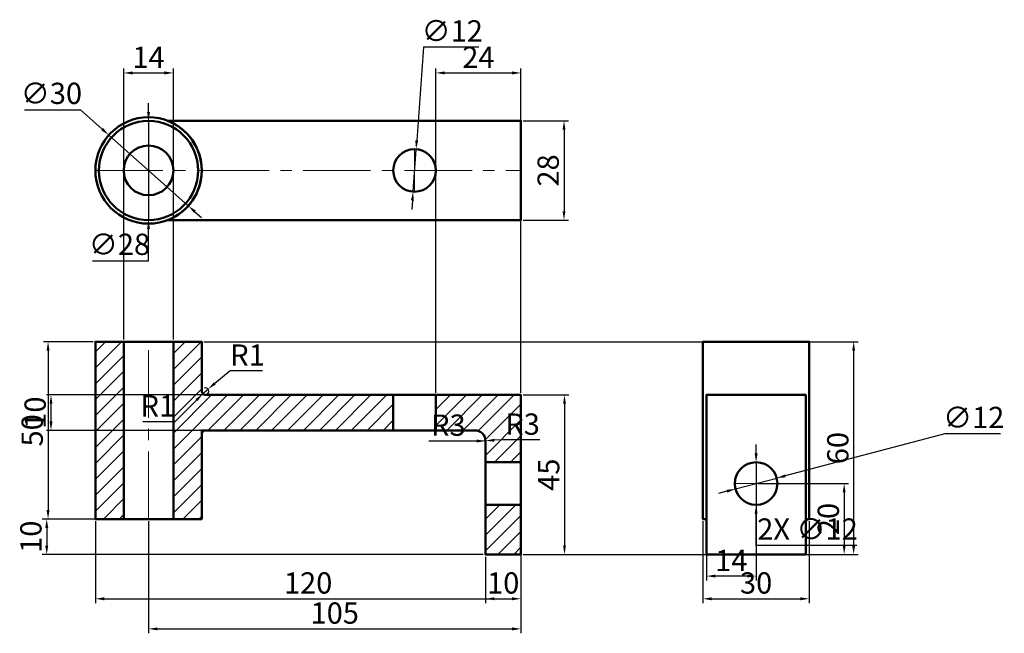
# Model space of a CAD drawing. Units: millimetres. Extents: x 11 to 289, y -7 to 166.
import ezdxf

# ---------------------------------------------------------------- set-up
doc = ezdxf.new("R2010")
doc.units = ezdxf.units.MM
doc.linetypes.add('CENTER2', pattern=[28.575, 19.05, -3.175, 3.175, -3.175])
for name, color, linetype, lineweight in [('M-CNTR', 4, 'CENTER2', 18), ('M-DIMS', 2, 'Continuous', 25), ('M-HATC', 8, 'Continuous', 18), ('M-OUTL', 7, 'Continuous', 50)]:
    doc.layers.add(name, color=color, linetype=linetype, lineweight=lineweight)
doc.styles.get("Standard").update_dxf_attribs({"font": 'arial.ttf'})
doc.dimstyles.new('ISO-25', dxfattribs={"dimtxt": 6, "dimasz": 2.5, "dimexe": 1.25, "dimexo": 0.625, "dimtad": 1, "dimtoh": 1, "dimdec": 0, "dimtxsty": 'Standard', "dimcen": 2.5, "dimadec": 0, "dimazin": 0, "dimtfac": 1, "dimtdec": 0, "dimtmove": 0, "dimatfit": 3, "dimfxl": 1, "dimarcsym": 0})

# ---------------------------------------------------------------- blocks, each defined once
blk = doc.blocks.new('*D1')
at = {"layer": 'Defpoints', "color": 0, "transparency": 16777216}
for p in [(139.29, 47.57), (142.29, 47.57)]:
    blk.add_point(p, dxfattribs=at)
at = {"layer": 'M-DIMS', "color": 0, "lineweight": -2, "transparency": 16777216}
blk.add_line((126.36, 47.57), (139.79, 47.57), dxfattribs=at)
at = {"layer": 'M-DIMS', "color": 0, "transparency": 16777216}
blk.add_solid([(139.79, 47.99), (139.79, 47.15), (142.29, 47.57)], dxfattribs=at)
at = {"layer": 'M-DIMS', "color": 0, "transparency": 16777216, "insert": (131.83, 51.26), "char_height": 6, "attachment_point": 5}
blk.add_mtext('R3', dxfattribs=at)
blk = doc.blocks.new('*D2')
at = {"layer": 'Defpoints', "color": 0, "transparency": 16777216}
for p in [(63.29, 61.57), (64.06, 62.21)]:
    blk.add_point(p, dxfattribs=at)
at = {"layer": 'M-DIMS', "color": 0, "lineweight": -2, "transparency": 16777216}
for p, q in [((70.31, 67.39), (65.98, 63.8)), ((79.45, 67.39), (70.31, 67.39)), ((63.29, 61.57), (64.06, 62.21))]:
    blk.add_line(p, q, dxfattribs=at)
blk.add_arc((63.29, 61.57), 1, 305.8099, 111.2749, dxfattribs=at)
at = {"layer": 'M-DIMS', "color": 0, "transparency": 16777216}
blk.add_solid([(65.72, 64.12), (66.25, 63.48), (64.06, 62.21)], dxfattribs=at)
at = {"layer": 'M-DIMS', "color": 0, "transparency": 16777216, "insert": (75.19, 71.03), "char_height": 6, "attachment_point": 5}
blk.add_mtext('R1', dxfattribs=at)
blk = doc.blocks.new('*D3')
at = {"layer": 'Defpoints', "color": 0, "transparency": 16777216}
for p in [(47.29, 25.57), (152.29, 25.57), (152.29, -5.41)]:
    blk.add_point(p, dxfattribs=at)
at = {"layer": 'M-DIMS', "color": 0, "lineweight": -2, "transparency": 16777216}
for p, q in [((47.29, 24.95), (47.29, -6.66)), ((152.29, 24.95), (152.29, -6.66)), ((49.79, -5.41), (149.79, -5.41))]:
    blk.add_line(p, q, dxfattribs=at)
at = {"layer": 'M-DIMS', "color": 0, "transparency": 16777216}
for points in [[(49.79, -5), (49.79, -5.83), (47.29, -5.41)], [(149.79, -5), (149.79, -5.83), (152.29, -5.41)]]:
    blk.add_solid(points, dxfattribs=at)
at = {"layer": 'M-DIMS', "color": 0, "transparency": 16777216, "insert": (99.79, -1.73), "char_height": 6, "attachment_point": 5}
blk.add_mtext('105', dxfattribs=at)
blk = doc.blocks.new('*D4')
at = {"layer": 'Defpoints', "color": 0, "transparency": 16777216}
for p in [(62.29, 25.57), (18.59, 15.57), (142.29, 15.57)]:
    blk.add_point(p, dxfattribs=at)
at = {"layer": 'M-DIMS', "color": 0, "lineweight": -2, "transparency": 16777216}
for p, q in [((61.66, 25.57), (17.34, 25.57)), ((18.59, 23.07), (18.59, 18.07)), ((141.66, 15.57), (17.34, 15.57))]:
    blk.add_line(p, q, dxfattribs=at)
at = {"layer": 'M-DIMS', "color": 0, "transparency": 16777216}
for points in [[(18.17, 23.07), (19.01, 23.07), (18.59, 25.57)], [(18.17, 18.07), (19.01, 18.07), (18.59, 15.57)]]:
    blk.add_solid(points, dxfattribs=at)
at = {"layer": 'M-DIMS', "color": 0, "transparency": 16777216, "insert": (14.9, 20.57), "char_height": 6, "attachment_point": 5, "rotation": 90}
blk.add_mtext('10', dxfattribs=at)
blk = doc.blocks.new('*D5')
at = {"layer": 'Defpoints', "color": 0, "transparency": 16777216}
for p in [(32.29, 75.57), (18.96, 25.57), (32.29, 25.57)]:
    blk.add_point(p, dxfattribs=at)
at = {"layer": 'M-DIMS', "color": 0, "lineweight": -2, "transparency": 16777216}
for p, q in [((31.66, 75.57), (17.71, 75.57)), ((18.96, 73.07), (18.96, 28.07)), ((31.66, 25.57), (17.71, 25.57))]:
    blk.add_line(p, q, dxfattribs=at)
at = {"layer": 'M-DIMS', "color": 0, "transparency": 16777216}
for points in [[(18.54, 73.07), (19.38, 73.07), (18.96, 75.57)], [(18.54, 28.07), (19.38, 28.07), (18.96, 25.57)]]:
    blk.add_solid(points, dxfattribs=at)
at = {"layer": 'M-DIMS', "color": 0, "transparency": 16777216, "insert": (15.27, 50.57), "char_height": 6, "attachment_point": 5, "rotation": 90}
blk.add_mtext('50', dxfattribs=at)
blk = doc.blocks.new('*D6')
at = {"layer": 'Defpoints', "color": 0, "transparency": 16777216}
for p in [(152.29, 60.57), (152.29, 15.57), (164.57, 15.57)]:
    blk.add_point(p, dxfattribs=at)
at = {"layer": 'M-DIMS', "color": 0, "lineweight": -2, "transparency": 16777216}
for p, q in [((152.91, 60.57), (165.82, 60.57)), ((164.57, 58.07), (164.57, 18.07)), ((152.91, 15.57), (165.82, 15.57))]:
    blk.add_line(p, q, dxfattribs=at)
at = {"layer": 'M-DIMS', "color": 0, "transparency": 16777216}
for points in [[(164.15, 58.07), (164.98, 58.07), (164.57, 60.57)], [(164.15, 18.07), (164.98, 18.07), (164.57, 15.57)]]:
    blk.add_solid(points, dxfattribs=at)
at = {"layer": 'M-DIMS', "color": 0, "transparency": 16777216, "insert": (160.89, 38.07), "char_height": 6, "attachment_point": 5, "rotation": 90}
blk.add_mtext('45', dxfattribs=at)
blk = doc.blocks.new('*D7')
at = {"layer": 'Defpoints', "color": 0, "transparency": 16777216}
for p in [(204.59, 35.57), (218.59, 35.57), (204.59, 9.47)]:
    blk.add_point(p, dxfattribs=at)
at = {"layer": 'M-DIMS', "color": 0, "lineweight": -2, "transparency": 16777216}
for p, q in [((204.59, 34.95), (204.59, 8.22)), ((218.59, 34.95), (218.59, 8.22)), ((216.09, 9.47), (207.09, 9.47))]:
    blk.add_line(p, q, dxfattribs=at)
at = {"layer": 'M-DIMS', "color": 0, "transparency": 16777216}
for points in [[(207.09, 9.89), (207.09, 9.06), (204.59, 9.47)], [(216.09, 9.89), (216.09, 9.06), (218.59, 9.47)]]:
    blk.add_solid(points, dxfattribs=at)
at = {"layer": 'M-DIMS', "color": 0, "transparency": 16777216, "insert": (211.59, 13.11), "char_height": 6, "attachment_point": 5}
blk.add_mtext('14', dxfattribs=at)
blk = doc.blocks.new('*D8')
at = {"layer": 'Defpoints', "color": 0, "transparency": 16777216}
for p in [(218.59, 35.57), (218.59, 15.57), (243.41, 15.57)]:
    blk.add_point(p, dxfattribs=at)
at = {"layer": 'M-DIMS', "color": 0, "lineweight": -2, "transparency": 16777216}
for p, q in [((219.21, 35.57), (244.66, 35.57)), ((243.41, 33.07), (243.41, 18.07)), ((219.21, 15.57), (244.66, 15.57))]:
    blk.add_line(p, q, dxfattribs=at)
at = {"layer": 'M-DIMS', "color": 0, "transparency": 16777216}
for points in [[(243, 33.07), (243.83, 33.07), (243.41, 35.57)], [(243, 18.07), (243.83, 18.07), (243.41, 15.57)]]:
    blk.add_solid(points, dxfattribs=at)
at = {"layer": 'M-DIMS', "color": 0, "transparency": 16777216, "insert": (239.72, 25.57), "char_height": 6, "attachment_point": 5, "rotation": 90}
blk.add_mtext('20', dxfattribs=at)
blk = doc.blocks.new('*D9')
at = {"layer": 'Defpoints', "color": 0, "transparency": 16777216}
for p in [(152.29, 137.87), (152.29, 109.87), (164.43, 109.87)]:
    blk.add_point(p, dxfattribs=at)
at = {"layer": 'M-DIMS', "color": 0, "lineweight": -2, "transparency": 16777216}
for p, q in [((152.91, 137.87), (165.68, 137.87)), ((164.43, 135.37), (164.43, 112.37)), ((152.91, 109.87), (165.68, 109.87))]:
    blk.add_line(p, q, dxfattribs=at)
at = {"layer": 'M-DIMS', "color": 0, "transparency": 16777216}
for points in [[(164.01, 135.37), (164.84, 135.37), (164.43, 137.87)], [(164.01, 112.37), (164.84, 112.37), (164.43, 109.87)]]:
    blk.add_solid(points, dxfattribs=at)
at = {"layer": 'M-DIMS', "color": 0, "transparency": 16777216, "insert": (160.74, 123.87), "char_height": 6, "attachment_point": 5, "rotation": 90}
blk.add_mtext('28', dxfattribs=at)
blk = doc.blocks.new('*D10')
at = {"layer": 'Defpoints', "color": 0, "transparency": 16777216}
for p in [(122.72, 129.86), (121.86, 117.89)]:
    blk.add_point(p, dxfattribs=at)
at = {"layer": 'M-DIMS', "color": 0, "lineweight": -2, "transparency": 16777216}
for p, q in [((124.77, 158.59), (122.89, 132.35)), ((140.45, 158.59), (124.77, 158.59)), ((121.86, 117.89), (122.72, 129.86)), ((121.68, 115.39), (121.5, 112.9))]:
    blk.add_line(p, q, dxfattribs=at)
at = {"layer": 'M-DIMS', "color": 0, "transparency": 16777216}
for points in [[(122.48, 132.38), (123.31, 132.32), (122.72, 129.86)], [(121.27, 115.42), (122.1, 115.36), (121.86, 117.89)]]:
    blk.add_solid(points, dxfattribs=at)
at = {"layer": 'M-DIMS', "color": 0, "transparency": 16777216, "insert": (132.92, 162.45), "char_height": 6, "attachment_point": 5}
blk.add_mtext('∅12', dxfattribs=at)
blk = doc.blocks.new('*D11')
at = {"layer": 'Defpoints', "color": 0, "transparency": 16777216}
for p in [(224.39, 37.1), (212.78, 34.04)]:
    blk.add_point(p, dxfattribs=at)
at = {"layer": 'M-DIMS', "color": 0, "lineweight": -2, "transparency": 16777216}
for p, q in [((271.77, 49.58), (226.81, 37.73)), ((287.46, 49.58), (271.77, 49.58)), ((212.78, 34.04), (224.39, 37.1)), ((210.37, 33.41), (207.95, 32.77))]:
    blk.add_line(p, q, dxfattribs=at)
at = {"layer": 'M-DIMS', "color": 0, "transparency": 16777216}
for points in [[(226.7, 38.14), (226.91, 37.33), (224.39, 37.1)], [(210.26, 33.81), (210.47, 33), (212.78, 34.04)]]:
    blk.add_solid(points, dxfattribs=at)
at = {"layer": 'M-DIMS', "color": 0, "transparency": 16777216, "insert": (279.93, 53.43), "char_height": 6, "attachment_point": 5}
blk.add_mtext('∅12', dxfattribs=at)
blk = doc.blocks.new('*D12')
at = {"layer": 'Defpoints', "color": 0, "transparency": 16777216}
for p in [(36.09, 133.85), (58.49, 113.9)]:
    blk.add_point(p, dxfattribs=at)
at = {"layer": 'M-DIMS', "color": 0, "lineweight": -2, "transparency": 16777216}
for p, q in [((12.36, 140.97), (28.08, 140.97)), ((28.08, 140.97), (34.22, 135.51)), ((58.49, 113.9), (36.09, 133.85)), ((60.36, 112.23), (62.23, 110.57))]:
    blk.add_line(p, q, dxfattribs=at)
at = {"layer": 'M-DIMS', "color": 0, "transparency": 16777216}
for points in [[(34.5, 135.82), (33.94, 135.2), (36.09, 133.85)], [(60.64, 112.54), (60.08, 111.92), (58.49, 113.9)]]:
    blk.add_solid(points, dxfattribs=at)
at = {"layer": 'M-DIMS', "color": 0, "transparency": 16777216, "insert": (19.91, 144.83), "char_height": 6, "attachment_point": 5}
blk.add_mtext('∅30', dxfattribs=at)
blk = doc.blocks.new('*D13')
at = {"layer": 'Defpoints', "color": 0, "transparency": 16777216}
for p in [(32.29, 25.57), (152.29, 15.57), (152.29, 3.07)]:
    blk.add_point(p, dxfattribs=at)
at = {"layer": 'M-DIMS', "color": 0, "lineweight": -2, "transparency": 16777216}
for p, q in [((32.29, 24.95), (32.29, 1.82)), ((152.29, 14.95), (152.29, 1.82)), ((34.79, 3.07), (149.79, 3.07))]:
    blk.add_line(p, q, dxfattribs=at)
at = {"layer": 'M-DIMS', "color": 0, "transparency": 16777216}
for points in [[(34.79, 3.49), (34.79, 2.65), (32.29, 3.07)], [(149.79, 3.49), (149.79, 2.65), (152.29, 3.07)]]:
    blk.add_solid(points, dxfattribs=at)
at = {"layer": 'M-DIMS', "color": 0, "transparency": 16777216, "insert": (92.29, 6.76), "char_height": 6, "attachment_point": 5}
blk.add_mtext('120', dxfattribs=at)
blk = doc.blocks.new('*D14')
at = {"layer": 'Defpoints', "color": 0, "transparency": 16777216}
for p in [(62.29, 75.57), (152.29, 15.57), (246.09, 15.57)]:
    blk.add_point(p, dxfattribs=at)
at = {"layer": 'M-DIMS', "color": 0, "lineweight": -2, "transparency": 16777216}
for p, q in [((62.91, 75.57), (247.34, 75.57)), ((246.09, 73.07), (246.09, 18.07)), ((152.91, 15.57), (247.34, 15.57))]:
    blk.add_line(p, q, dxfattribs=at)
at = {"layer": 'M-DIMS', "color": 0, "transparency": 16777216}
for points in [[(245.67, 73.07), (246.5, 73.07), (246.09, 75.57)], [(245.67, 18.07), (246.5, 18.07), (246.09, 15.57)]]:
    blk.add_solid(points, dxfattribs=at)
at = {"layer": 'M-DIMS', "color": 0, "transparency": 16777216, "insert": (242.4, 45.57), "char_height": 6, "attachment_point": 5, "rotation": 90}
blk.add_mtext('60', dxfattribs=at)
blk = doc.blocks.new('*D15')
at = {"layer": 'Defpoints', "color": 0, "transparency": 16777216}
for p in [(152.29, 151.37), (128.29, 60.57), (152.29, 60.57)]:
    blk.add_point(p, dxfattribs=at)
at = {"layer": 'M-DIMS', "color": 0, "lineweight": -2, "transparency": 16777216}
for p, q in [((128.29, 61.2), (128.29, 152.62)), ((130.79, 151.37), (149.79, 151.37)), ((152.29, 61.2), (152.29, 152.62))]:
    blk.add_line(p, q, dxfattribs=at)
at = {"layer": 'M-DIMS', "color": 0, "transparency": 16777216}
for points in [[(130.79, 151.79), (130.79, 150.95), (128.29, 151.37)], [(149.79, 151.79), (149.79, 150.95), (152.29, 151.37)]]:
    blk.add_solid(points, dxfattribs=at)
at = {"layer": 'M-DIMS', "color": 0, "transparency": 16777216, "insert": (140.29, 155.01), "char_height": 6, "attachment_point": 5}
blk.add_mtext('24', dxfattribs=at)
blk = doc.blocks.new('*D16')
at = {"layer": 'Defpoints', "color": 0, "transparency": 16777216}
for p in [(54.29, 151.37), (40.29, 75.57), (54.29, 75.57)]:
    blk.add_point(p, dxfattribs=at)
at = {"layer": 'M-DIMS', "color": 0, "lineweight": -2, "transparency": 16777216}
for p, q in [((40.29, 76.2), (40.29, 152.62)), ((42.79, 151.37), (51.79, 151.37)), ((54.29, 76.2), (54.29, 152.62))]:
    blk.add_line(p, q, dxfattribs=at)
at = {"layer": 'M-DIMS', "color": 0, "transparency": 16777216}
for points in [[(42.79, 151.79), (42.79, 150.95), (40.29, 151.37)], [(51.79, 151.79), (51.79, 150.95), (54.29, 151.37)]]:
    blk.add_solid(points, dxfattribs=at)
at = {"layer": 'M-DIMS', "color": 0, "transparency": 16777216, "insert": (47.29, 155.01), "char_height": 6, "attachment_point": 5}
blk.add_mtext('14', dxfattribs=at)
blk = doc.blocks.new('*D17')
at = {"layer": 'Defpoints', "color": 0, "transparency": 16777216}
for p in [(203.59, 25.57), (233.59, 25.57), (233.59, 3.07)]:
    blk.add_point(p, dxfattribs=at)
at = {"layer": 'M-DIMS', "color": 0, "lineweight": -2, "transparency": 16777216}
for p, q in [((203.59, 24.95), (203.59, 1.82)), ((233.59, 24.95), (233.59, 1.82)), ((206.09, 3.07), (231.09, 3.07))]:
    blk.add_line(p, q, dxfattribs=at)
at = {"layer": 'M-DIMS', "color": 0, "transparency": 16777216}
for points in [[(206.09, 3.49), (206.09, 2.65), (203.59, 3.07)], [(231.09, 3.49), (231.09, 2.65), (233.59, 3.07)]]:
    blk.add_solid(points, dxfattribs=at)
at = {"layer": 'M-DIMS', "color": 0, "transparency": 16777216, "insert": (218.59, 6.76), "char_height": 6, "attachment_point": 5}
blk.add_mtext('30', dxfattribs=at)
blk = doc.blocks.new('*D18')
at = {"layer": 'Defpoints', "color": 0, "transparency": 16777216}
for p in [(116.29, 60.57), (19.79, 50.57), (116.29, 50.57)]:
    blk.add_point(p, dxfattribs=at)
at = {"layer": 'M-DIMS', "color": 0, "lineweight": -2, "transparency": 16777216}
for p, q in [((115.66, 60.57), (18.54, 60.57)), ((19.79, 58.07), (19.79, 53.07)), ((115.66, 50.57), (18.54, 50.57))]:
    blk.add_line(p, q, dxfattribs=at)
at = {"layer": 'M-DIMS', "color": 0, "transparency": 16777216}
for points in [[(19.37, 58.07), (20.2, 58.07), (19.79, 60.57)], [(19.37, 53.07), (20.2, 53.07), (19.79, 50.57)]]:
    blk.add_solid(points, dxfattribs=at)
at = {"layer": 'M-DIMS', "color": 0, "transparency": 16777216, "insert": (16.1, 55.57), "char_height": 6, "attachment_point": 5, "rotation": 90}
blk.add_mtext('10', dxfattribs=at)
blk = doc.blocks.new('*D19')
at = {"layer": 'Defpoints', "color": 0, "transparency": 16777216}
for p in [(142.29, 15.57), (152.29, 15.57), (152.29, 3.07)]:
    blk.add_point(p, dxfattribs=at)
at = {"layer": 'M-DIMS', "color": 0, "lineweight": -2, "transparency": 16777216}
for p, q in [((142.29, 14.95), (142.29, 1.82)), ((152.29, 14.95), (152.29, 1.82)), ((144.79, 3.07), (149.79, 3.07))]:
    blk.add_line(p, q, dxfattribs=at)
at = {"layer": 'M-DIMS', "color": 0, "transparency": 16777216}
for points in [[(144.79, 3.49), (144.79, 2.65), (142.29, 3.07)], [(149.79, 3.49), (149.79, 2.65), (152.29, 3.07)]]:
    blk.add_solid(points, dxfattribs=at)
at = {"layer": 'M-DIMS', "color": 0, "transparency": 16777216, "insert": (147.29, 6.76), "char_height": 6, "attachment_point": 5}
blk.add_mtext('10', dxfattribs=at)
blk = doc.blocks.new('*D20')
at = {"layer": 'Defpoints', "color": 0, "transparency": 16777216}
for p in [(47.29, 137.87), (47.29, 109.87)]:
    blk.add_point(p, dxfattribs=at)
at = {"layer": 'M-DIMS', "color": 0, "lineweight": -2, "transparency": 16777216}
for p, q in [((47.29, 140.37), (47.29, 142.87)), ((47.29, 137.87), (47.29, 109.87)), ((47.29, 98.41), (47.29, 107.37)), ((31.53, 98.41), (47.29, 98.41))]:
    blk.add_line(p, q, dxfattribs=at)
at = {"layer": 'M-DIMS', "color": 0, "transparency": 16777216}
for points in [[(46.87, 140.37), (47.71, 140.37), (47.29, 137.87)], [(46.87, 107.37), (47.7, 107.37), (47.29, 109.87)]]:
    blk.add_solid(points, dxfattribs=at)
at = {"layer": 'M-DIMS', "color": 0, "transparency": 16777216, "insert": (39.1, 102.26), "char_height": 6, "attachment_point": 5}
blk.add_mtext('∅28', dxfattribs=at)
blk = doc.blocks.new('*D21')
at = {"layer": 'Defpoints', "color": 0, "transparency": 16777216}
for p in [(218.59, 41.57), (218.59, 29.57)]:
    blk.add_point(p, dxfattribs=at)
at = {"layer": 'M-DIMS', "color": 0, "lineweight": -2, "transparency": 16777216}
for p, q in [((218.59, 44.07), (218.59, 46.57)), ((218.59, 41.57), (218.59, 29.57)), ((218.59, 18.11), (218.59, 27.07)), ((246.95, 18.11), (218.59, 18.11))]:
    blk.add_line(p, q, dxfattribs=at)
at = {"layer": 'M-DIMS', "color": 0, "transparency": 16777216}
for points in [[(219, 44.07), (218.17, 44.07), (218.59, 41.57)], [(219, 27.07), (218.17, 27.07), (218.59, 29.57)]]:
    blk.add_solid(points, dxfattribs=at)
at = {"layer": 'M-DIMS', "color": 0, "transparency": 16777216, "insert": (233.08, 21.96), "char_height": 6, "attachment_point": 5}
blk.add_mtext('2X ∅12', dxfattribs=at)
blk = doc.blocks.new('*D22')
at = {"layer": 'Defpoints', "color": 0, "transparency": 16777216}
for p in [(139.29, 47.57), (142.29, 47.68)]:
    blk.add_point(p, dxfattribs=at)
at = {"layer": 'M-DIMS', "color": 0, "lineweight": -2, "transparency": 16777216}
for p, q in [((139.29, 47.57), (142.29, 47.68)), ((147.28, 47.86), (144.78, 47.77)), ((157.58, 47.86), (147.28, 47.86))]:
    blk.add_line(p, q, dxfattribs=at)
at = {"layer": 'M-DIMS', "color": 0, "transparency": 16777216}
blk.add_solid([(144.77, 48.19), (144.8, 47.35), (142.29, 47.68)], dxfattribs=at)
at = {"layer": 'M-DIMS', "color": 0, "transparency": 16777216, "insert": (152.75, 51.55), "char_height": 6, "attachment_point": 5}
blk.add_mtext('R3', dxfattribs=at)
blk = doc.blocks.new('*D23')
at = {"layer": 'Defpoints', "color": 0, "transparency": 16777216}
for p in [(63.29, 61.57), (62.58, 60.86)]:
    blk.add_point(p, dxfattribs=at)
at = {"layer": 'M-DIMS', "color": 0, "lineweight": -2, "transparency": 16777216}
for p, q in [((63.29, 61.57), (62.58, 60.86)), ((54.8, 53.06), (60.82, 59.09)), ((45.66, 53.06), (54.8, 53.06))]:
    blk.add_line(p, q, dxfattribs=at)
at = {"layer": 'M-DIMS', "color": 0, "transparency": 16777216}
blk.add_solid([(60.52, 59.39), (61.11, 58.8), (62.58, 60.86)], dxfattribs=at)
at = {"layer": 'M-DIMS', "color": 0, "transparency": 16777216, "insert": (49.91, 56.69), "char_height": 6, "attachment_point": 5}
blk.add_mtext('R1', dxfattribs=at)

msp = doc.modelspace()

# ---------------------------------------------------------------- hatches: boundary and pattern name
at = {"layer": 'M-HATC'}
h = msp.add_hatch(dxfattribs=at)
h.set_pattern_fill('ANSI31', color=256)
h.paths.add_polyline_path([(40.29, 75.57), (32.29, 75.57), (32.29, 25.57), (40.29, 25.57)])
h.paths.add_polyline_path([(116.29, 60.57), (63.29, 60.57, -0.414214), (62.29, 61.57), (62.29, 75.57), (54.29, 75.57), (54.29, 25.57), (62.29, 25.57), (62.29, 49.57), (62.29, 50.57), (63.29, 50.57), (116.29, 50.57)])
h.paths.add_polyline_path([(152.29, 60.57), (128.29, 60.57), (128.29, 50.57), (139.29, 50.57, -0.414214), (142.29, 47.57), (142.29, 41.57), (152.29, 41.57)])
h.paths.add_polyline_path([(152.29, 29.57), (142.29, 29.57), (142.29, 15.57), (152.29, 15.57)])

# ---------------------------------------------------------------- linework, layer by layer
at = {"layer": 'M-CNTR'}
for p, q in [((47.29, 138.87), (47.29, 108.87)), ((122.29, 129.87), (122.29, 117.87)), ((47.29, 25.57), (47.29, 75.57)), ((218.59, 41.57), (218.59, 29.57)), ((212.59, 35.57), (224.59, 35.57))]:
    msp.add_line(p, q, dxfattribs=at)
msp.add_lwpolyline([(32.29, 123.87), (62.29, 123.87), (152.29, 123.87)], dxfattribs=at)
at = {"layer": 'M-OUTL'}
for p, q in [((40.29, 25.57), (40.29, 75.57)), ((54.29, 25.57), (54.29, 75.57)), ((116.29, 60.57), (116.29, 50.57)), ((128.29, 60.57), (128.29, 50.57)), ((152.29, 41.57), (142.29, 41.57)), ((152.29, 29.57), (142.29, 29.57))]:
    msp.add_line(p, q, dxfattribs=at)
for points in [[(52.67, 137.87), (152.29, 137.87), (152.29, 109.87), (52.67, 109.87)], [(204.59, 25.57), (204.59, 15.57), (232.59, 15.57), (232.59, 60.57), (204.59, 60.57), (204.59, 25.57), (203.59, 25.57), (203.59, 75.57), (233.59, 75.57), (233.59, 25.57), (232.59, 25.57)]]:
    msp.add_lwpolyline(points, dxfattribs=at)
msp.add_lwpolyline([(62.29, 49.57, -0.414214), (63.29, 50.57), (62.29, 50.57), (62.29, 49.57), (62.29, 25.57), (32.29, 25.57), (32.29, 75.57), (62.29, 75.57), (62.29, 61.57, 0.414214), (63.29, 60.57), (152.29, 60.57), (152.29, 15.57), (142.29, 15.57), (142.29, 47.57, 0.414214), (139.29, 50.57), (63.29, 50.57)], format="xyb", dxfattribs=at)
for centre, radius in [((47.29, 123.87), 15), ((47.29, 123.87), 14), ((47.29, 123.87), 7), ((122.29, 123.87), 6), ((218.59, 35.57), 6)]:
    msp.add_circle(centre, radius, dxfattribs=at)
msp.add_arc((47.29, 123.87), 15, 291.0395, 68.9605, dxfattribs=at)

# ---------------------------------------------------------------- dimensions: what is measured, and where the dimension line sits
at = {"layer": 'M-DIMS'}
for p1, p2, override, picture, middle in [((121.86, 117.89), (122.72, 129.86), {"dimclrd": 0, "dimclre": 0, "dimclrt": 0}, '*D10', (132.92, 158.59)), ((58.49, 113.9), (36.09, 133.85), {"dimclrd": 0, "dimclre": 0, "dimclrt": 0}, '*D12', (19.91, 140.97)), ((47.29, 137.87), (47.29, 109.87), {"dimdec": 0, "dimlfac": 1, "dimrnd": 0, "dimzin": 0, "dimdsep": 46, "dimlunit": 2}, '*D20', (39.1, 98.41)), ((212.78, 34.04), (224.39, 37.1), {"dimclrd": 0, "dimclre": 0, "dimclrt": 0}, '*D11', (271.77, 49.58))]:
    dim = msp.add_diameter_dim_2p(p1=p1, p2=p2, dimstyle='ISO-25', override=override, dxfattribs=at)
    dim.commit()
    dim.dimension.update_dxf_attribs({"geometry": picture, "text_midpoint": middle, "dimtype": 163})
for base, p1, p2, override, picture, middle in [((54.29, 151.37), (40.29, 75.57), (54.29, 75.57), {"dimdec": 0, "dimlfac": 1, "dimrnd": 0, "dimzin": 0, "dimdsep": 46, "dimlunit": 2}, '*D16', (47.29, 155.01)), ((152.29, 151.37), (128.29, 60.57), (152.29, 60.57), {"dimdec": 0, "dimlfac": 1, "dimrnd": 0, "dimzin": 0, "dimdsep": 46, "dimlunit": 2}, '*D15', (140.29, 155.01)), ((204.59, 9.47), (218.59, 35.57), (204.59, 35.57), {"dimclrd": 0, "dimclre": 0, "dimclrt": 0}, '*D7', (211.59, 13.11)), ((152.29, 3.07), (32.29, 25.57), (152.29, 15.57), {"dimdec": 0, "dimlfac": 1, "dimrnd": 0, "dimzin": 0, "dimdsep": 46, "dimlunit": 2}, '*D13', (92.29, 6.76)), ((152.29, -5.41), (47.29, 25.57), (152.29, 25.57), {"dimclrd": 0, "dimclre": 0, "dimclrt": 0}, '*D3', (99.79, -1.73)), ((233.59, 3.07), (203.59, 25.57), (233.59, 25.57), {"dimdec": 0, "dimlfac": 1, "dimrnd": 0, "dimzin": 0, "dimdsep": 46, "dimlunit": 2}, '*D17', (218.59, 6.76)), ((152.29, 3.07), (142.29, 15.57), (152.29, 15.57), {"dimdec": 0, "dimlfac": 1, "dimrnd": 0, "dimzin": 0, "dimdsep": 46, "dimlunit": 2}, '*D19', (147.29, 6.76))]:
    dim = msp.add_linear_dim(base=base, p1=p1, p2=p2, dimstyle='ISO-25', override=override, dxfattribs=at)
    dim.commit()
    dim.dimension.update_dxf_attribs({"geometry": picture, "text_midpoint": middle})
for base, p1, p2, override, picture, middle in [((164.43, 109.87), (152.29, 137.87), (152.29, 109.87), {"dimclrd": 0, "dimclre": 0, "dimclrt": 0}, '*D9', (160.74, 123.87)), ((18.96, 25.57), (32.29, 75.57), (32.29, 25.57), {"dimclrd": 0, "dimclre": 0, "dimclrt": 0}, '*D5', (15.27, 50.57)), ((246.09, 15.57), (62.29, 75.57), (152.29, 15.57), {"dimdec": 0, "dimlfac": 1, "dimrnd": 0, "dimzin": 0, "dimdsep": 46, "dimlunit": 2}, '*D14', (242.4, 45.57)), ((19.79, 50.57), (116.29, 60.57), (116.29, 50.57), {"dimdec": 0, "dimlfac": 1, "dimrnd": 0, "dimzin": 0, "dimdsep": 46, "dimlunit": 2}, '*D18', (16.1, 55.57)), ((164.57, 15.57), (152.29, 60.57), (152.29, 15.57), {"dimclrd": 0, "dimclre": 0, "dimclrt": 0}, '*D6', (160.89, 38.07)), ((243.41, 15.57), (218.59, 35.57), (218.59, 15.57), {"dimclrd": 0, "dimclre": 0, "dimclrt": 0}, '*D8', (239.72, 25.57)), ((18.59, 15.57), (62.29, 25.57), (142.29, 15.57), {"dimclrd": 0, "dimclre": 0, "dimclrt": 0}, '*D4', (14.9, 20.57))]:
    dim = msp.add_linear_dim(base=base, p1=p1, p2=p2, angle=90, dimstyle='ISO-25', override=override, dxfattribs=at)
    dim.commit()
    dim.dimension.update_dxf_attribs({"geometry": picture, "text_midpoint": middle})
for center, mpoint, picture, middle in [((63.29, 61.57), (64.06, 62.21), '*D2', (75.19, 67.39)), ((139.29, 47.57), (142.29, 47.57), '*D1', (131.83, 47.57))]:
    dim = msp.add_radius_dim(center=center, mpoint=mpoint, dimstyle='ISO-25', override={"dimclrd": 0, "dimclre": 0, "dimclrt": 0}, dxfattribs=at)
    dim.commit()
    dim.dimension.update_dxf_attribs({"geometry": picture, "text_midpoint": middle, "dimtype": 164})
for center, mpoint, picture, middle in [((63.29, 61.57), (62.58, 60.86), '*D23', (49.91, 56.69)), ((139.29, 47.57), (142.29, 47.68), '*D22', (152.75, 51.55))]:
    dim = msp.add_radius_dim(center=center, mpoint=mpoint, dimstyle='ISO-25', override={"dimdec": 0, "dimlfac": 1, "dimrnd": 0, "dimzin": 0, "dimdsep": 46, "dimlunit": 2}, dxfattribs=at)
    dim.commit()
    dim.dimension.update_dxf_attribs({"geometry": picture, "text_midpoint": middle})
dim = msp.add_diameter_dim_2p(p1=(218.59, 41.57), p2=(218.59, 29.57), text='2X <>', dimstyle='ISO-25', override={"dimdec": 0, "dimlfac": 1, "dimrnd": 0, "dimzin": 0, "dimdsep": 46, "dimlunit": 2}, dxfattribs=at)
dim.commit()
dim.dimension.update_dxf_attribs({"geometry": '*D21', "text_midpoint": (233.08, 18.11), "dimtype": 163})

doc.saveas('drawing.dxf')
